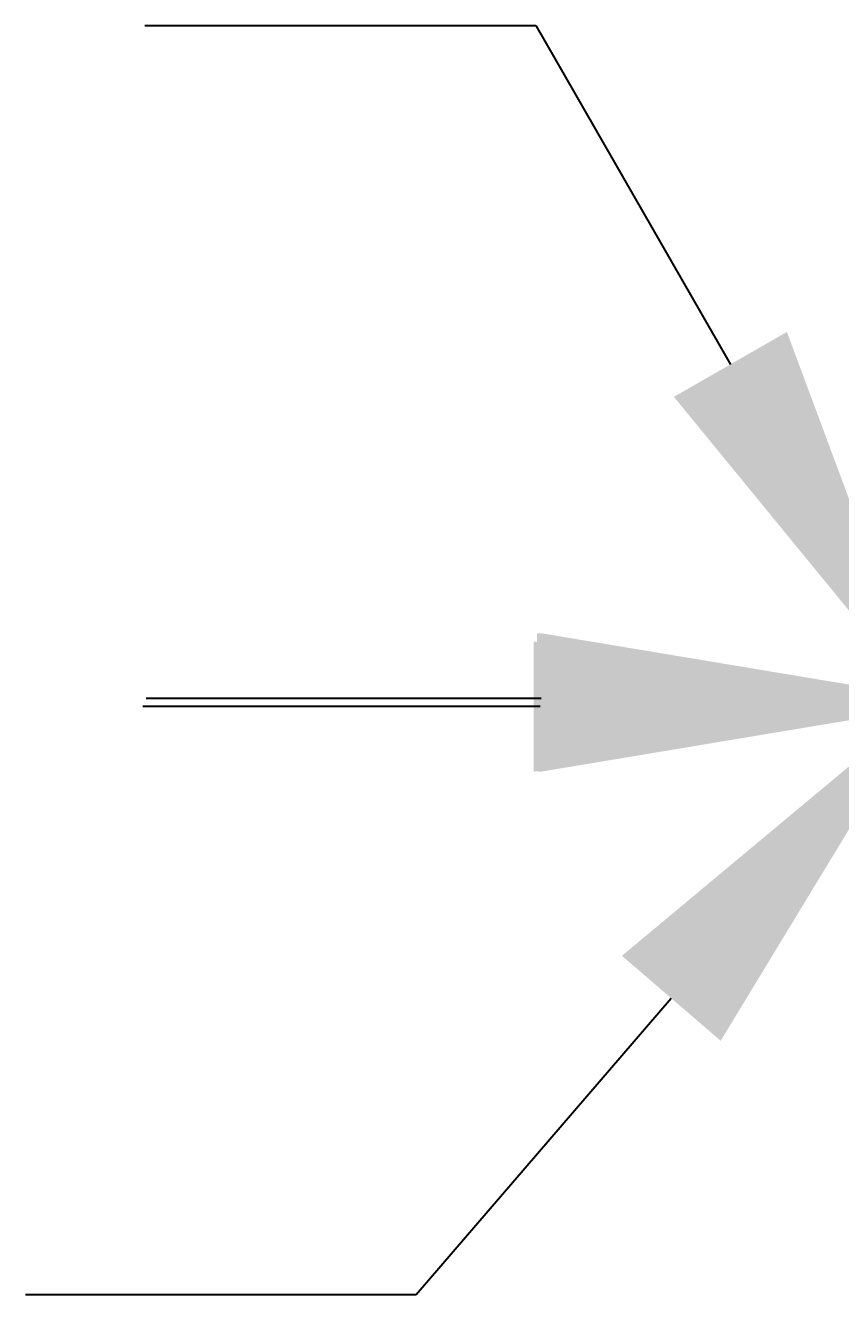
# Model space of a CAD drawing. Units: millimetres. Extents: x -22994 to 29398, y -19990 to 20176.
# Tile 1 of 135: x -22994 to -2139, y -15047 to 17422. Entities that reach past the tile are written whole.
import ezdxf

# ---------------------------------------------------------------- set-up
doc = ezdxf.new("R2010")
doc.units = ezdxf.units.MM
doc.header["$MEASUREMENT"] = 0
doc.layers.add('M-DIMS', color=2, linetype='Continuous', lineweight=18)
doc.styles.get("Standard").update_dxf_attribs({"font": 'arial.ttf'})
doc.dimstyles.get("Standard").update_dxf_attribs({"dimtxt": 0.18, "dimasz": 10000, "dimexe": 0.18, "dimexo": 0.0625, "dimgap": 0.09, "dimtad": 0, "dimtih": 1, "dimtoh": 1, "dimdec": 0, "dimzin": 0, "dimdsep": 46, "dimtxsty": 'Standard', "dimcen": 0.09, "dimadec": 0, "dimazin": 0, "dimtfac": 1, "dimtdec": 0, "dimtofl": 0, "dimtmove": 0, "dimatfit": 3, "dimfxl": 1, "dimtolj": 1, "dimtzin": 0, "dimlwd": 30, "dimarcsym": 0})

# ---------------------------------------------------------------- blocks, each defined once
blk = doc.blocks.new('*D2')
at = {"layer": 'Defpoints', "color": 0, "transparency": 16777216}
for p in [(7, 10), (291, 10), (291, -5)]:
    blk.add_point(p, dxfattribs=at)
at = {"layer": 'M-DIMS', "color": 0, "lineweight": -2, "transparency": 16777216}
for p, q in [((7, 10), (7, -5)), ((291, 10), (291, -5))]:
    blk.add_line(p, q, dxfattribs=at)
at = {"layer": 'M-DIMS', "color": 0, "lineweight": 30, "transparency": 16777216}
for p, q in [((-9993, -5), (-19993, -5)), ((10291, -5), (20291, -5))]:
    blk.add_line(p, q, dxfattribs=at)
at = {"layer": 'M-DIMS', "color": 0, "transparency": 16777216}
for points in [[(-9993, 1662), (-9993, -1672), (7, -5)], [(10291, 1662), (10291, -1672), (291, -5)]]:
    blk.add_solid(points, dxfattribs=at)
at = {"layer": 'M-DIMS', "color": 0, "transparency": 16777216, "insert": (149, -5), "char_height": 0.18, "attachment_point": 5}
blk.add_mtext('\\A1;284.2', dxfattribs=at)
blk = doc.blocks.new('*D3')
at = {"layer": 'Defpoints', "color": 0, "transparency": 16777216}
for p in [(96, 128), (110, 204), (110, 176)]:
    blk.add_point(p, dxfattribs=at)
at = {"layer": 'M-DIMS', "color": 0, "lineweight": 30, "transparency": 16777216}
for p, q in [((-9904, 204), (-19904, 204)), ((10110, 204), (20110, 204))]:
    blk.add_line(p, q, dxfattribs=at)
at = {"layer": 'M-DIMS', "color": 0, "lineweight": -2, "transparency": 16777216}
for p, q in [((96, 128), (96, 204)), ((110, 176), (110, 204))]:
    blk.add_line(p, q, dxfattribs=at)
at = {"layer": 'M-DIMS', "color": 0, "transparency": 16777216}
for points in [[(-9904, 1871), (-9904, -1463), (96, 204)], [(10110, 1871), (10110, -1463), (110, 204)]]:
    blk.add_solid(points, dxfattribs=at)
at = {"layer": 'M-DIMS', "color": 0, "transparency": 16777216, "insert": (103, 204), "char_height": 0.18, "attachment_point": 5}
blk.add_mtext('\\A1;14.432', dxfattribs=at)
blk = doc.blocks.new('*D4')
at = {"layer": 'Defpoints', "color": 0, "transparency": 16777216}
for p in [(110, 176), (116, 204), (116, 176)]:
    blk.add_point(p, dxfattribs=at)
at = {"layer": 'M-DIMS', "color": 0, "lineweight": 30, "transparency": 16777216}
for p, q in [((-9890, 204), (-19890, 204)), ((10116, 204), (20116, 204))]:
    blk.add_line(p, q, dxfattribs=at)
at = {"layer": 'M-DIMS', "color": 0, "lineweight": -2, "transparency": 16777216}
for p, q in [((110, 176), (110, 204)), ((116, 176), (116, 204))]:
    blk.add_line(p, q, dxfattribs=at)
at = {"layer": 'M-DIMS', "color": 0, "transparency": 16777216}
for points in [[(-9890, 1871), (-9890, -1463), (110, 204)], [(10116, 1871), (10116, -1463), (116, 204)]]:
    blk.add_solid(points, dxfattribs=at)
at = {"layer": 'M-DIMS', "color": 0, "transparency": 16777216, "insert": (113, 204), "char_height": 0.18, "attachment_point": 5}
blk.add_mtext('\\A1;6', dxfattribs=at)
blk = doc.blocks.new('*D5')
at = {"layer": 'Defpoints', "color": 0, "transparency": 16777216}
for p in [(116, 176), (181, 204), (181, 176)]:
    blk.add_point(p, dxfattribs=at)
at = {"layer": 'M-DIMS', "color": 0, "lineweight": 30, "transparency": 16777216}
for p, q in [((-9884, 204), (-19884, 204)), ((10181, 204), (20181, 204))]:
    blk.add_line(p, q, dxfattribs=at)
at = {"layer": 'M-DIMS', "color": 0, "lineweight": -2, "transparency": 16777216}
for p, q in [((116, 176), (116, 204)), ((181, 176), (181, 204))]:
    blk.add_line(p, q, dxfattribs=at)
at = {"layer": 'M-DIMS', "color": 0, "transparency": 16777216}
for points in [[(-9884, 1871), (-9884, -1463), (116, 204)], [(10181, 1871), (10181, -1463), (181, 204)]]:
    blk.add_solid(points, dxfattribs=at)
at = {"layer": 'M-DIMS', "color": 0, "transparency": 16777216, "insert": (149, 204), "char_height": 0.18, "attachment_point": 5}
blk.add_mtext('\\A1;65', dxfattribs=at)
blk = doc.blocks.new('*D6')
at = {"layer": 'Defpoints', "color": 0, "transparency": 16777216}
for p in [(181, 176), (187, 204), (187, 176)]:
    blk.add_point(p, dxfattribs=at)
at = {"layer": 'M-DIMS', "color": 0, "lineweight": 30, "transparency": 16777216}
for p, q in [((-9819, 204), (-19819, 204)), ((10187, 204), (20187, 204))]:
    blk.add_line(p, q, dxfattribs=at)
at = {"layer": 'M-DIMS', "color": 0, "lineweight": -2, "transparency": 16777216}
for p, q in [((181, 176), (181, 204)), ((187, 176), (187, 204))]:
    blk.add_line(p, q, dxfattribs=at)
at = {"layer": 'M-DIMS', "color": 0, "transparency": 16777216}
for points in [[(-9819, 1871), (-9819, -1463), (181, 204)], [(10187, 1871), (10187, -1463), (187, 204)]]:
    blk.add_solid(points, dxfattribs=at)
at = {"layer": 'M-DIMS', "color": 0, "transparency": 16777216, "insert": (184, 204), "char_height": 0.18, "attachment_point": 5}
blk.add_mtext('\\A1;6', dxfattribs=at)
blk = doc.blocks.new('*D7')
at = {"layer": 'Defpoints', "color": 0, "transparency": 16777216}
for p in [(187, 176), (202, 204), (202, 128)]:
    blk.add_point(p, dxfattribs=at)
at = {"layer": 'M-DIMS', "color": 0, "lineweight": 30, "transparency": 16777216}
for p, q in [((-9813, 204), (-19813, 204)), ((10202, 204), (20202, 204))]:
    blk.add_line(p, q, dxfattribs=at)
at = {"layer": 'M-DIMS', "color": 0, "lineweight": -2, "transparency": 16777216}
for p, q in [((187, 176), (187, 204)), ((202, 128), (202, 204))]:
    blk.add_line(p, q, dxfattribs=at)
at = {"layer": 'M-DIMS', "color": 0, "transparency": 16777216}
for points in [[(-9813, 1871), (-9813, -1463), (187, 204)], [(10202, 1871), (10202, -1463), (202, 204)]]:
    blk.add_solid(points, dxfattribs=at)
at = {"layer": 'M-DIMS', "color": 0, "transparency": 16777216, "insert": (194, 204), "char_height": 0.18, "attachment_point": 5}
blk.add_mtext('\\A1;14.432', dxfattribs=at)
blk = doc.blocks.new('*D8')
at = {"layer": 'Defpoints', "color": 0, "transparency": 16777216}
for p in [(202, 128), (228, 204), (228, 147)]:
    blk.add_point(p, dxfattribs=at)
at = {"layer": 'M-DIMS', "color": 0, "lineweight": 30, "transparency": 16777216}
for p, q in [((-9798, 204), (-19798, 204)), ((10228, 204), (20228, 204))]:
    blk.add_line(p, q, dxfattribs=at)
at = {"layer": 'M-DIMS', "color": 0, "lineweight": -2, "transparency": 16777216}
for p, q in [((202, 128), (202, 204)), ((228, 147), (228, 204))]:
    blk.add_line(p, q, dxfattribs=at)
at = {"layer": 'M-DIMS', "color": 0, "transparency": 16777216}
for points in [[(-9798, 1871), (-9798, -1463), (202, 204)], [(10228, 1871), (10228, -1463), (228, 204)]]:
    blk.add_solid(points, dxfattribs=at)
at = {"layer": 'M-DIMS', "color": 0, "transparency": 16777216, "insert": (215, 204), "char_height": 0.18, "attachment_point": 5}
blk.add_mtext('\\A1;25.95', dxfattribs=at)
blk = doc.blocks.new('*D10')
at = {"layer": 'Defpoints', "color": 0, "transparency": 16777216}
for p in [(126, 136), (133, 136), (133, -5)]:
    blk.add_point(p, dxfattribs=at)
at = {"layer": 'M-DIMS', "color": 0, "lineweight": -2, "transparency": 16777216}
for p, q in [((126, 136), (126, -5)), ((133, 136), (133, -5))]:
    blk.add_line(p, q, dxfattribs=at)
at = {"layer": 'M-DIMS', "color": 0, "lineweight": 30, "transparency": 16777216}
for p, q in [((-9874, -5), (-19874, -5)), ((10133, -5), (20133, -5))]:
    blk.add_line(p, q, dxfattribs=at)
at = {"layer": 'M-DIMS', "color": 0, "transparency": 16777216}
for points in [[(-9874, 1662), (-9874, -1672), (126, -5)], [(10133, 1662), (10133, -1672), (133, -5)]]:
    blk.add_solid(points, dxfattribs=at)
at = {"layer": 'M-DIMS', "color": 0, "transparency": 16777216, "insert": (129, -5), "char_height": 0.18, "attachment_point": 5}
blk.add_mtext('\\A1;7.696', dxfattribs=at)
blk = doc.blocks.new('*D11')
at = {"layer": 'Defpoints', "color": 0, "transparency": 16777216}
for p in [(133, 136), (136, 136), (136, -5)]:
    blk.add_point(p, dxfattribs=at)
at = {"layer": 'M-DIMS', "color": 0, "lineweight": -2, "transparency": 16777216}
for p, q in [((133, 136), (133, -5)), ((136, 136), (136, -5))]:
    blk.add_line(p, q, dxfattribs=at)
at = {"layer": 'M-DIMS', "color": 0, "lineweight": 30, "transparency": 16777216}
for p, q in [((-9867, -5), (-19867, -5)), ((10136, -5), (20136, -5))]:
    blk.add_line(p, q, dxfattribs=at)
at = {"layer": 'M-DIMS', "color": 0, "transparency": 16777216}
for points in [[(-9867, 1662), (-9867, -1672), (133, -5)], [(10136, 1662), (10136, -1672), (136, -5)]]:
    blk.add_solid(points, dxfattribs=at)
at = {"layer": 'M-DIMS', "color": 0, "transparency": 16777216, "insert": (134, -5), "char_height": 0.18, "attachment_point": 5}
blk.add_mtext('\\A1;2.304', dxfattribs=at)
blk = doc.blocks.new('*D12')
at = {"layer": 'Defpoints', "color": 0, "transparency": 16777216}
for p in [(136, 136), (146, 136), (146, -5)]:
    blk.add_point(p, dxfattribs=at)
at = {"layer": 'M-DIMS', "color": 0, "lineweight": -2, "transparency": 16777216}
for p, q in [((136, 136), (136, -5)), ((146, 136), (146, -5))]:
    blk.add_line(p, q, dxfattribs=at)
at = {"layer": 'M-DIMS', "color": 0, "lineweight": 30, "transparency": 16777216}
for p, q in [((-9864, -5), (-19864, -5)), ((10146, -5), (20146, -5))]:
    blk.add_line(p, q, dxfattribs=at)
at = {"layer": 'M-DIMS', "color": 0, "transparency": 16777216}
for points in [[(-9864, 1662), (-9864, -1672), (136, -5)], [(10146, 1662), (10146, -1672), (146, -5)]]:
    blk.add_solid(points, dxfattribs=at)
at = {"layer": 'M-DIMS', "color": 0, "transparency": 16777216, "insert": (141, -5), "char_height": 0.18, "attachment_point": 5}
blk.add_mtext('\\A1;10', dxfattribs=at)
blk = doc.blocks.new('*D13')
at = {"layer": 'Defpoints', "color": 0, "transparency": 16777216}
for p in [(146, 136), (156, 136), (156, -5)]:
    blk.add_point(p, dxfattribs=at)
at = {"layer": 'M-DIMS', "color": 0, "lineweight": -2, "transparency": 16777216}
for p, q in [((146, 136), (146, -5)), ((156, 136), (156, -5))]:
    blk.add_line(p, q, dxfattribs=at)
at = {"layer": 'M-DIMS', "color": 0, "lineweight": 30, "transparency": 16777216}
for p, q in [((-9854, -5), (-19854, -5)), ((10156, -5), (20156, -5))]:
    blk.add_line(p, q, dxfattribs=at)
at = {"layer": 'M-DIMS', "color": 0, "transparency": 16777216}
for points in [[(-9854, 1662), (-9854, -1672), (146, -5)], [(10156, 1662), (10156, -1672), (156, -5)]]:
    blk.add_solid(points, dxfattribs=at)
at = {"layer": 'M-DIMS', "color": 0, "transparency": 16777216, "insert": (151, -5), "char_height": 0.18, "attachment_point": 5}
blk.add_mtext('\\A1;10', dxfattribs=at)
blk = doc.blocks.new('*D14')
at = {"layer": 'Defpoints', "color": 0, "transparency": 16777216}
for p in [(156, 136), (166, 136), (166, -5)]:
    blk.add_point(p, dxfattribs=at)
at = {"layer": 'M-DIMS', "color": 0, "lineweight": -2, "transparency": 16777216}
for p, q in [((156, 136), (156, -5)), ((166, 136), (166, -5))]:
    blk.add_line(p, q, dxfattribs=at)
at = {"layer": 'M-DIMS', "color": 0, "lineweight": 30, "transparency": 16777216}
for p, q in [((-9844, -5), (-19844, -5)), ((10166, -5), (20166, -5))]:
    blk.add_line(p, q, dxfattribs=at)
at = {"layer": 'M-DIMS', "color": 0, "transparency": 16777216}
for points in [[(-9844, 1662), (-9844, -1672), (156, -5)], [(10166, 1662), (10166, -1672), (166, -5)]]:
    blk.add_solid(points, dxfattribs=at)
at = {"layer": 'M-DIMS', "color": 0, "transparency": 16777216, "insert": (161, -5), "char_height": 0.18, "attachment_point": 5}
blk.add_mtext('\\A1;10', dxfattribs=at)
blk = doc.blocks.new('*D16')
at = {"layer": 'Defpoints', "color": 0, "transparency": 16777216}
for p in [(110, 48), (120, 204), (120, 48)]:
    blk.add_point(p, dxfattribs=at)
at = {"layer": 'M-DIMS', "color": 0, "lineweight": 30, "transparency": 16777216}
for p, q in [((-9890, 204), (-19890, 204)), ((10120, 204), (20120, 204))]:
    blk.add_line(p, q, dxfattribs=at)
at = {"layer": 'M-DIMS', "color": 0, "lineweight": -2, "transparency": 16777216}
for p, q in [((110, 48), (110, 204)), ((120, 48), (120, 204))]:
    blk.add_line(p, q, dxfattribs=at)
at = {"layer": 'M-DIMS', "color": 0, "transparency": 16777216}
for points in [[(-9890, 1871), (-9890, -1463), (110, 204)], [(10120, 1871), (10120, -1463), (120, 204)]]:
    blk.add_solid(points, dxfattribs=at)
at = {"layer": 'M-DIMS', "color": 0, "transparency": 16777216, "insert": (115, 204), "char_height": 0.18, "attachment_point": 5}
blk.add_mtext('\\A1;9.704', dxfattribs=at)
blk = doc.blocks.new('*D17')
at = {"layer": 'Defpoints', "color": 0, "transparency": 16777216}
for p in [(120, 48), (126, 204), (126, 48)]:
    blk.add_point(p, dxfattribs=at)
at = {"layer": 'M-DIMS', "color": 0, "lineweight": 30, "transparency": 16777216}
for p, q in [((-9880, 204), (-19880, 204)), ((10126, 204), (20126, 204))]:
    blk.add_line(p, q, dxfattribs=at)
at = {"layer": 'M-DIMS', "color": 0, "lineweight": -2, "transparency": 16777216}
for p, q in [((120, 48), (120, 204)), ((126, 48), (126, 204))]:
    blk.add_line(p, q, dxfattribs=at)
at = {"layer": 'M-DIMS', "color": 0, "transparency": 16777216}
for points in [[(-9880, 1871), (-9880, -1463), (120, 204)], [(10126, 1871), (10126, -1463), (126, 204)]]:
    blk.add_solid(points, dxfattribs=at)
at = {"layer": 'M-DIMS', "color": 0, "transparency": 16777216, "insert": (123, 204), "char_height": 0.18, "attachment_point": 5}
blk.add_mtext('\\A1;6', dxfattribs=at)
blk = doc.blocks.new('*D18')
at = {"layer": 'Defpoints', "color": 0, "transparency": 16777216}
for p in [(126, 48), (132, 204), (132, 48)]:
    blk.add_point(p, dxfattribs=at)
at = {"layer": 'M-DIMS', "color": 0, "lineweight": 30, "transparency": 16777216}
for p, q in [((-9874, 204), (-19874, 204)), ((10132, 204), (20132, 204))]:
    blk.add_line(p, q, dxfattribs=at)
at = {"layer": 'M-DIMS', "color": 0, "lineweight": -2, "transparency": 16777216}
for p, q in [((126, 48), (126, 204)), ((132, 48), (132, 204))]:
    blk.add_line(p, q, dxfattribs=at)
at = {"layer": 'M-DIMS', "color": 0, "transparency": 16777216}
for points in [[(-9874, 1871), (-9874, -1463), (126, 204)], [(10132, 1871), (10132, -1463), (132, 204)]]:
    blk.add_solid(points, dxfattribs=at)
at = {"layer": 'M-DIMS', "color": 0, "transparency": 16777216, "insert": (129, 204), "char_height": 0.18, "attachment_point": 5}
blk.add_mtext('\\A1;6', dxfattribs=at)
blk = doc.blocks.new('*D19')
at = {"layer": 'Defpoints', "color": 0, "transparency": 16777216}
for p in [(132, 48), (138, 204), (138, 48)]:
    blk.add_point(p, dxfattribs=at)
at = {"layer": 'M-DIMS', "color": 0, "lineweight": 30, "transparency": 16777216}
for p, q in [((-9868, 204), (-19868, 204)), ((10138, 204), (20138, 204))]:
    blk.add_line(p, q, dxfattribs=at)
at = {"layer": 'M-DIMS', "color": 0, "lineweight": -2, "transparency": 16777216}
for p, q in [((132, 48), (132, 204)), ((138, 48), (138, 204))]:
    blk.add_line(p, q, dxfattribs=at)
at = {"layer": 'M-DIMS', "color": 0, "transparency": 16777216}
for points in [[(-9868, 1871), (-9868, -1463), (132, 204)], [(10138, 1871), (10138, -1463), (138, 204)]]:
    blk.add_solid(points, dxfattribs=at)
at = {"layer": 'M-DIMS', "color": 0, "transparency": 16777216, "insert": (135, 204), "char_height": 0.18, "attachment_point": 5}
blk.add_mtext('\\A1;6', dxfattribs=at)
blk = doc.blocks.new('*D20')
at = {"layer": 'Defpoints', "color": 0, "transparency": 16777216}
for p in [(138, 48), (144, 204), (144, 48)]:
    blk.add_point(p, dxfattribs=at)
at = {"layer": 'M-DIMS', "color": 0, "lineweight": 30, "transparency": 16777216}
for p, q in [((-9862, 204), (-19862, 204)), ((10144, 204), (20144, 204))]:
    blk.add_line(p, q, dxfattribs=at)
at = {"layer": 'M-DIMS', "color": 0, "lineweight": -2, "transparency": 16777216}
for p, q in [((138, 48), (138, 204)), ((144, 48), (144, 204))]:
    blk.add_line(p, q, dxfattribs=at)
at = {"layer": 'M-DIMS', "color": 0, "transparency": 16777216}
for points in [[(-9862, 1871), (-9862, -1463), (138, 204)], [(10144, 1871), (10144, -1463), (144, 204)]]:
    blk.add_solid(points, dxfattribs=at)
at = {"layer": 'M-DIMS', "color": 0, "transparency": 16777216, "insert": (141, 204), "char_height": 0.18, "attachment_point": 5}
blk.add_mtext('\\A1;6', dxfattribs=at)
blk = doc.blocks.new('*D21')
at = {"layer": 'Defpoints', "color": 0, "transparency": 16777216}
for p in [(144, 48), (149, 204), (149, 48)]:
    blk.add_point(p, dxfattribs=at)
at = {"layer": 'M-DIMS', "color": 0, "lineweight": 30, "transparency": 16777216}
for p, q in [((-9856, 204), (-19856, 204)), ((10149, 204), (20149, 204))]:
    blk.add_line(p, q, dxfattribs=at)
at = {"layer": 'M-DIMS', "color": 0, "lineweight": -2, "transparency": 16777216}
for p, q in [((144, 48), (144, 204)), ((149, 48), (149, 204))]:
    blk.add_line(p, q, dxfattribs=at)
at = {"layer": 'M-DIMS', "color": 0, "transparency": 16777216}
for points in [[(-9856, 1871), (-9856, -1463), (144, 204)], [(10149, 1871), (10149, -1463), (149, 204)]]:
    blk.add_solid(points, dxfattribs=at)
at = {"layer": 'M-DIMS', "color": 0, "transparency": 16777216, "insert": (147, 204), "char_height": 0.18, "attachment_point": 5}
blk.add_mtext('\\A1;4.945', dxfattribs=at)
blk = doc.blocks.new('*D22')
at = {"layer": 'Defpoints', "color": 0, "transparency": 16777216}
for p in [(149, 31), (155, 31), (155, -5)]:
    blk.add_point(p, dxfattribs=at)
at = {"layer": 'M-DIMS', "color": 0, "lineweight": -2, "transparency": 16777216}
for p, q in [((149, 31), (149, -5)), ((155, 31), (155, -5))]:
    blk.add_line(p, q, dxfattribs=at)
at = {"layer": 'M-DIMS', "color": 0, "lineweight": 30, "transparency": 16777216}
for p, q in [((-9851, -5), (-19851, -5)), ((10155, -5), (20155, -5))]:
    blk.add_line(p, q, dxfattribs=at)
at = {"layer": 'M-DIMS', "color": 0, "transparency": 16777216}
for points in [[(-9851, 1662), (-9851, -1672), (149, -5)], [(10155, 1662), (10155, -1672), (155, -5)]]:
    blk.add_solid(points, dxfattribs=at)
at = {"layer": 'M-DIMS', "color": 0, "transparency": 16777216, "insert": (152, -5), "char_height": 0.18, "attachment_point": 5}
blk.add_mtext('\\A1;6', dxfattribs=at)
blk = doc.blocks.new('*D23')
at = {"layer": 'Defpoints', "color": 0, "transparency": 16777216}
for p in [(155, 31), (161, 31), (161, -5)]:
    blk.add_point(p, dxfattribs=at)
at = {"layer": 'M-DIMS', "color": 0, "lineweight": -2, "transparency": 16777216}
for p, q in [((155, 31), (155, -5)), ((161, 31), (161, -5))]:
    blk.add_line(p, q, dxfattribs=at)
at = {"layer": 'M-DIMS', "color": 0, "lineweight": 30, "transparency": 16777216}
for p, q in [((-9845, -5), (-19845, -5)), ((10161, -5), (20161, -5))]:
    blk.add_line(p, q, dxfattribs=at)
at = {"layer": 'M-DIMS', "color": 0, "transparency": 16777216}
for points in [[(-9845, 1662), (-9845, -1672), (155, -5)], [(10161, 1662), (10161, -1672), (161, -5)]]:
    blk.add_solid(points, dxfattribs=at)
at = {"layer": 'M-DIMS', "color": 0, "transparency": 16777216, "insert": (158, -5), "char_height": 0.18, "attachment_point": 5}
blk.add_mtext('\\A1;6', dxfattribs=at)
blk = doc.blocks.new('*D24')
at = {"layer": 'Defpoints', "color": 0, "transparency": 16777216}
for p in [(161, 31), (166, 31), (166, -5)]:
    blk.add_point(p, dxfattribs=at)
at = {"layer": 'M-DIMS', "color": 0, "lineweight": -2, "transparency": 16777216}
for p, q in [((161, 31), (161, -5)), ((166, 31), (166, -5))]:
    blk.add_line(p, q, dxfattribs=at)
at = {"layer": 'M-DIMS', "color": 0, "lineweight": 30, "transparency": 16777216}
for p, q in [((-9839, -5), (-19839, -5)), ((10166, -5), (20166, -5))]:
    blk.add_line(p, q, dxfattribs=at)
at = {"layer": 'M-DIMS', "color": 0, "transparency": 16777216}
for points in [[(-9839, 1662), (-9839, -1672), (161, -5)], [(10166, 1662), (10166, -1672), (166, -5)]]:
    blk.add_solid(points, dxfattribs=at)
at = {"layer": 'M-DIMS', "color": 0, "transparency": 16777216, "insert": (164, -5), "char_height": 0.18, "attachment_point": 5}
blk.add_mtext('\\A1;5.323', dxfattribs=at)
blk = doc.blocks.new('*D25')
at = {"layer": 'Defpoints', "color": 0, "transparency": 16777216}
for p in [(166, 31), (172, 31), (172, -5)]:
    blk.add_point(p, dxfattribs=at)
at = {"layer": 'M-DIMS', "color": 0, "lineweight": -2, "transparency": 16777216}
for p, q in [((166, 31), (166, -5)), ((172, 31), (172, -5))]:
    blk.add_line(p, q, dxfattribs=at)
at = {"layer": 'M-DIMS', "color": 0, "lineweight": 30, "transparency": 16777216}
for p, q in [((-9834, -5), (-19834, -5)), ((10172, -5), (20172, -5))]:
    blk.add_line(p, q, dxfattribs=at)
at = {"layer": 'M-DIMS', "color": 0, "transparency": 16777216}
for points in [[(-9834, 1662), (-9834, -1672), (166, -5)], [(10172, 1662), (10172, -1672), (172, -5)]]:
    blk.add_solid(points, dxfattribs=at)
at = {"layer": 'M-DIMS', "color": 0, "transparency": 16777216, "insert": (169, -5), "char_height": 0.18, "attachment_point": 5}
blk.add_mtext('\\A1;6', dxfattribs=at)
blk = doc.blocks.new('*D26')
at = {"layer": 'Defpoints', "color": 0, "transparency": 16777216}
for p in [(172, 31), (178, 31), (178, -5)]:
    blk.add_point(p, dxfattribs=at)
at = {"layer": 'M-DIMS', "color": 0, "lineweight": -2, "transparency": 16777216}
for p, q in [((172, 31), (172, -5)), ((178, 31), (178, -5))]:
    blk.add_line(p, q, dxfattribs=at)
at = {"layer": 'M-DIMS', "color": 0, "lineweight": 30, "transparency": 16777216}
for p, q in [((-9828, -5), (-19828, -5)), ((10178, -5), (20178, -5))]:
    blk.add_line(p, q, dxfattribs=at)
at = {"layer": 'M-DIMS', "color": 0, "transparency": 16777216}
for points in [[(-9828, 1662), (-9828, -1672), (172, -5)], [(10178, 1662), (10178, -1672), (178, -5)]]:
    blk.add_solid(points, dxfattribs=at)
at = {"layer": 'M-DIMS', "color": 0, "transparency": 16777216, "insert": (175, -5), "char_height": 0.18, "attachment_point": 5}
blk.add_mtext('\\A1;6', dxfattribs=at)
blk = doc.blocks.new('*D27')
at = {"layer": 'Defpoints', "color": 0, "transparency": 16777216}
for p in [(178, 31), (188, 31), (188, -5)]:
    blk.add_point(p, dxfattribs=at)
at = {"layer": 'M-DIMS', "color": 0, "lineweight": -2, "transparency": 16777216}
for p, q in [((178, 31), (178, -5)), ((188, 31), (188, -5))]:
    blk.add_line(p, q, dxfattribs=at)
at = {"layer": 'M-DIMS', "color": 0, "lineweight": 30, "transparency": 16777216}
for p, q in [((-9822, -5), (-19822, -5)), ((10188, -5), (20188, -5))]:
    blk.add_line(p, q, dxfattribs=at)
at = {"layer": 'M-DIMS', "color": 0, "transparency": 16777216}
for points in [[(-9822, 1662), (-9822, -1672), (178, -5)], [(10188, 1662), (10188, -1672), (188, -5)]]:
    blk.add_solid(points, dxfattribs=at)
at = {"layer": 'M-DIMS', "color": 0, "transparency": 16777216, "insert": (183, -5), "char_height": 0.18, "attachment_point": 5}
blk.add_mtext('\\A1;9.679', dxfattribs=at)
blk = doc.blocks.new('*D32')
at = {"layer": 'Defpoints', "color": 0, "transparency": 16777216}
for p in [(52, 113), (57, 119)]:
    blk.add_point(p, dxfattribs=at)
at = {"layer": 'M-DIMS', "color": 0, "lineweight": -2, "transparency": 16777216}
blk.add_line((57, 119), (57, 119), dxfattribs=at)
blk.add_line((57, 119), (57, 119), dxfattribs=at)
at = {"layer": 'M-DIMS', "color": 0, "lineweight": 30, "transparency": 16777216}
for p, q in [((-12993, -15047), (-6470, -7467)), ((-22993, -15047), (-12993, -15047))]:
    blk.add_line(p, q, dxfattribs=at)
at = {"layer": 'M-DIMS', "color": 0, "transparency": 16777216}
blk.add_solid([(-7733, -6380), (-5207, -8554), (52, 113)], dxfattribs=at)
at = {"layer": 'M-DIMS', "color": 0, "transparency": 16777216, "insert": (-22993, -15047), "char_height": 0.18, "attachment_point": 5}
blk.add_mtext('\\A1;2X R7.284', dxfattribs=at)
blk = doc.blocks.new('*D35')
at = {"layer": 'Defpoints', "color": 0, "transparency": 16777216}
for p in [(21, 77), (22, 76)]:
    blk.add_point(p, dxfattribs=at)
at = {"layer": 'M-DIMS', "color": 0, "lineweight": 30, "transparency": 16777216}
for p, q in [((-19938, 17421), (-9938, 17421)), ((-9938, 17421), (-4958, 8749))]:
    blk.add_line(p, q, dxfattribs=at)
at = {"layer": 'M-DIMS', "color": 0, "lineweight": -2, "transparency": 16777216}
blk.add_line((22, 76), (22, 76), dxfattribs=at)
blk.add_line((22, 76), (22, 76), dxfattribs=at)
at = {"layer": 'M-DIMS', "color": 0, "transparency": 16777216}
blk.add_solid([(-3513, 9579), (-6404, 7919), (21, 77)], dxfattribs=at)
at = {"layer": 'M-DIMS', "color": 0, "transparency": 16777216, "insert": (-19938, 17421), "char_height": 0.18, "attachment_point": 5}
blk.add_mtext('\\A1;R1.5', dxfattribs=at)

msp = doc.modelspace()

# ---------------------------------------------------------------- dimensions: what is measured, and where the dimension line sits
at = {"layer": 'M-DIMS'}
dim = msp.add_radius_dim(center=(21.8402, 76.0922), mpoint=(21.0933, 77.393), dimstyle='Standard', override={"dimdec": 1, "dimlfac": 1, "dimrnd": 0, "dimzin": 0, "dimdsep": 46, "dimlunit": 2}, dxfattribs=at)
dim.commit()
dim.dimension.update_dxf_attribs({"geometry": '*D35', "text_midpoint": (-19938.3541, 17421.4466)})
for base, p1, p2, override, picture, middle in [((290.852, -5.0787), (6.6773, 10.2713), (290.852, 10.2713), {"dimdec": 1, "dimlfac": 1, "dimrnd": 0, "dimzin": 0, "dimdsep": 46, "dimlunit": 2}, '*D2', (148.7647, -5.0787)), ((110.2647, 204.1654), (95.8327, 127.967), (110.2647, 176.3662), {"dimdec": 3, "dimlfac": 1, "dimrnd": 0, "dimzin": 0, "dimdsep": 46, "dimlunit": 2}, '*D3', (103.0487, 204.1654)), ((116.2647, 204.1654), (110.2647, 176.3662), (116.2647, 176.3662), {"dimdec": 0, "dimlfac": 1, "dimrnd": 0, "dimzin": 0, "dimdsep": 46, "dimlunit": 2}, '*D4', (113.2647, 204.1654)), ((120.1702, 204.1654), (110.4658, 48.0349), (120.1702, 48.0349), {"dimdec": 3, "dimlfac": 1, "dimrnd": 0, "dimzin": 0, "dimdsep": 46, "dimlunit": 2}, '*D16', (115.318, 204.1654)), ((181.2647, 204.1654), (116.2647, 176.3662), (181.2647, 176.3662), {"dimdec": 0, "dimlfac": 1, "dimrnd": 0, "dimzin": 0, "dimdsep": 46, "dimlunit": 2}, '*D5', (148.7647, 204.1654)), ((126.1702, 204.1654), (120.1702, 48.0349), (126.1702, 48.0349), {"dimdec": 0, "dimlfac": 1, "dimrnd": 0, "dimzin": 0, "dimdsep": 46, "dimlunit": 2}, '*D17', (123.1702, 204.1654)), ((133.3459, -5.0787), (125.6498, 136.0713), (133.3459, 136.0713), {"dimdec": 3, "dimlfac": 1, "dimrnd": 0, "dimzin": 0, "dimdsep": 46, "dimlunit": 2}, '*D10', (129.4978, -5.0787)), ((132.1702, 204.1654), (126.1702, 48.0349), (132.1702, 48.0349), {"dimdec": 0, "dimlfac": 1, "dimrnd": 0, "dimzin": 0, "dimdsep": 46, "dimlunit": 2}, '*D18', (129.1702, 204.1654)), ((138.1702, 204.1654), (132.1702, 48.0349), (138.1702, 48.0349), {"dimdec": 0, "dimlfac": 1, "dimrnd": 0, "dimzin": 0, "dimdsep": 46, "dimlunit": 2}, '*D19', (135.1702, 204.1654)), ((135.6498, -5.0787), (133.3459, 136.0713), (135.6498, 136.0713), {"dimdec": 3, "dimlfac": 1, "dimrnd": 0, "dimzin": 0, "dimdsep": 46, "dimlunit": 2}, '*D11', (134.4978, -5.0787)), ((145.6498, -5.0787), (135.6498, 136.0713), (145.6498, 136.0713), {"dimdec": 0, "dimlfac": 1, "dimrnd": 0, "dimzin": 0, "dimdsep": 46, "dimlunit": 2}, '*D12', (140.6498, -5.0787)), ((144.1702, 204.1654), (138.1702, 48.0349), (144.1702, 48.0349), {"dimdec": 0, "dimlfac": 1, "dimrnd": 0, "dimzin": 0, "dimdsep": 46, "dimlunit": 2}, '*D20', (141.1702, 204.1654)), ((149.11567, 204.16539), (144.17023, 48.03494), (149.11567, 48.03494), {"dimdec": 3, "dimlfac": 1, "dimrnd": 0, "dimzin": 0, "dimdsep": 46, "dimlunit": 2}, '*D21', (146.64295, 204.16539)), ((155.6498, -5.0787), (145.6498, 136.0713), (155.6498, 136.0713), {"dimdec": 0, "dimlfac": 1, "dimrnd": 0, "dimzin": 0, "dimdsep": 46, "dimlunit": 2}, '*D13', (150.6498, -5.0787)), ((155.1157, -5.0787), (149.1157, 30.9895), (155.1157, 30.9895), {"dimdec": 0, "dimlfac": 1, "dimrnd": 0, "dimzin": 0, "dimdsep": 46, "dimlunit": 2}, '*D22', (152.1157, -5.0787)), ((161.1157, -5.0787), (155.1157, 30.9895), (161.1157, 30.9895), {"dimdec": 0, "dimlfac": 1, "dimrnd": 0, "dimzin": 0, "dimdsep": 46, "dimlunit": 2}, '*D23', (158.1157, -5.0787)), ((165.6498, -5.0787), (155.6498, 136.0713), (165.6498, 136.0713), {"dimdec": 0, "dimlfac": 1, "dimrnd": 0, "dimzin": 0, "dimdsep": 46, "dimlunit": 2}, '*D14', (160.6498, -5.0787)), ((166.4387, -5.0787), (161.1157, 30.9895), (166.4387, 30.9895), {"dimdec": 3, "dimlfac": 1, "dimrnd": 0, "dimzin": 0, "dimdsep": 46, "dimlunit": 2}, '*D24', (163.7772, -5.0787)), ((172.4387, -5.0787), (166.4387, 30.9895), (172.4387, 30.9895), {"dimdec": 0, "dimlfac": 1, "dimrnd": 0, "dimzin": 0, "dimdsep": 46, "dimlunit": 2}, '*D25', (169.4387, -5.0787)), ((178.4387, -5.0787), (172.4387, 30.9895), (178.4387, 30.9895), {"dimdec": 0, "dimlfac": 1, "dimrnd": 0, "dimzin": 0, "dimdsep": 46, "dimlunit": 2}, '*D26', (175.4387, -5.0787)), ((188.1175, -5.0787), (178.4387, 30.9895), (188.1175, 30.9895), {"dimdec": 3, "dimlfac": 1, "dimrnd": 0, "dimzin": 0, "dimdsep": 46, "dimlunit": 2}, '*D27', (183.2781, -5.0787)), ((187.2647, 204.1654), (181.2647, 176.3662), (187.2647, 176.3662), {"dimdec": 0, "dimlfac": 1, "dimrnd": 0, "dimzin": 0, "dimdsep": 46, "dimlunit": 2}, '*D6', (184.2647, 204.1654)), ((201.6967, 204.1654), (187.2647, 176.3662), (201.6967, 127.967), {"dimdec": 3, "dimlfac": 1, "dimrnd": 0, "dimzin": 0, "dimdsep": 46, "dimlunit": 2}, '*D7', (194.4807, 204.1654)), ((227.6485, 204.1654), (201.6967, 127.967), (227.6485, 146.7296), {"dimdec": 2, "dimlfac": 1, "dimrnd": 0, "dimzin": 0, "dimdsep": 46, "dimlunit": 2}, '*D8', (214.6726, 204.1654))]:
    dim = msp.add_linear_dim(base=base, p1=p1, p2=p2, dimstyle='Standard', override=override, dxfattribs=at)
    dim.commit()
    dim.dimension.update_dxf_attribs({"geometry": picture, "text_midpoint": middle})
dim = msp.add_radius_dim(center=(57.1639, 118.6143), mpoint=(52.4129, 113.0929), text='2X <>', dimstyle='Standard', override={"dimdec": 3, "dimlfac": 1, "dimrnd": 0, "dimzin": 0, "dimdsep": 46, "dimlunit": 2}, dxfattribs=at)
dim.commit()
dim.dimension.update_dxf_attribs({"geometry": '*D32', "text_midpoint": (-22993.208, -15047.0314)})

doc.saveas('drawing.dxf')
